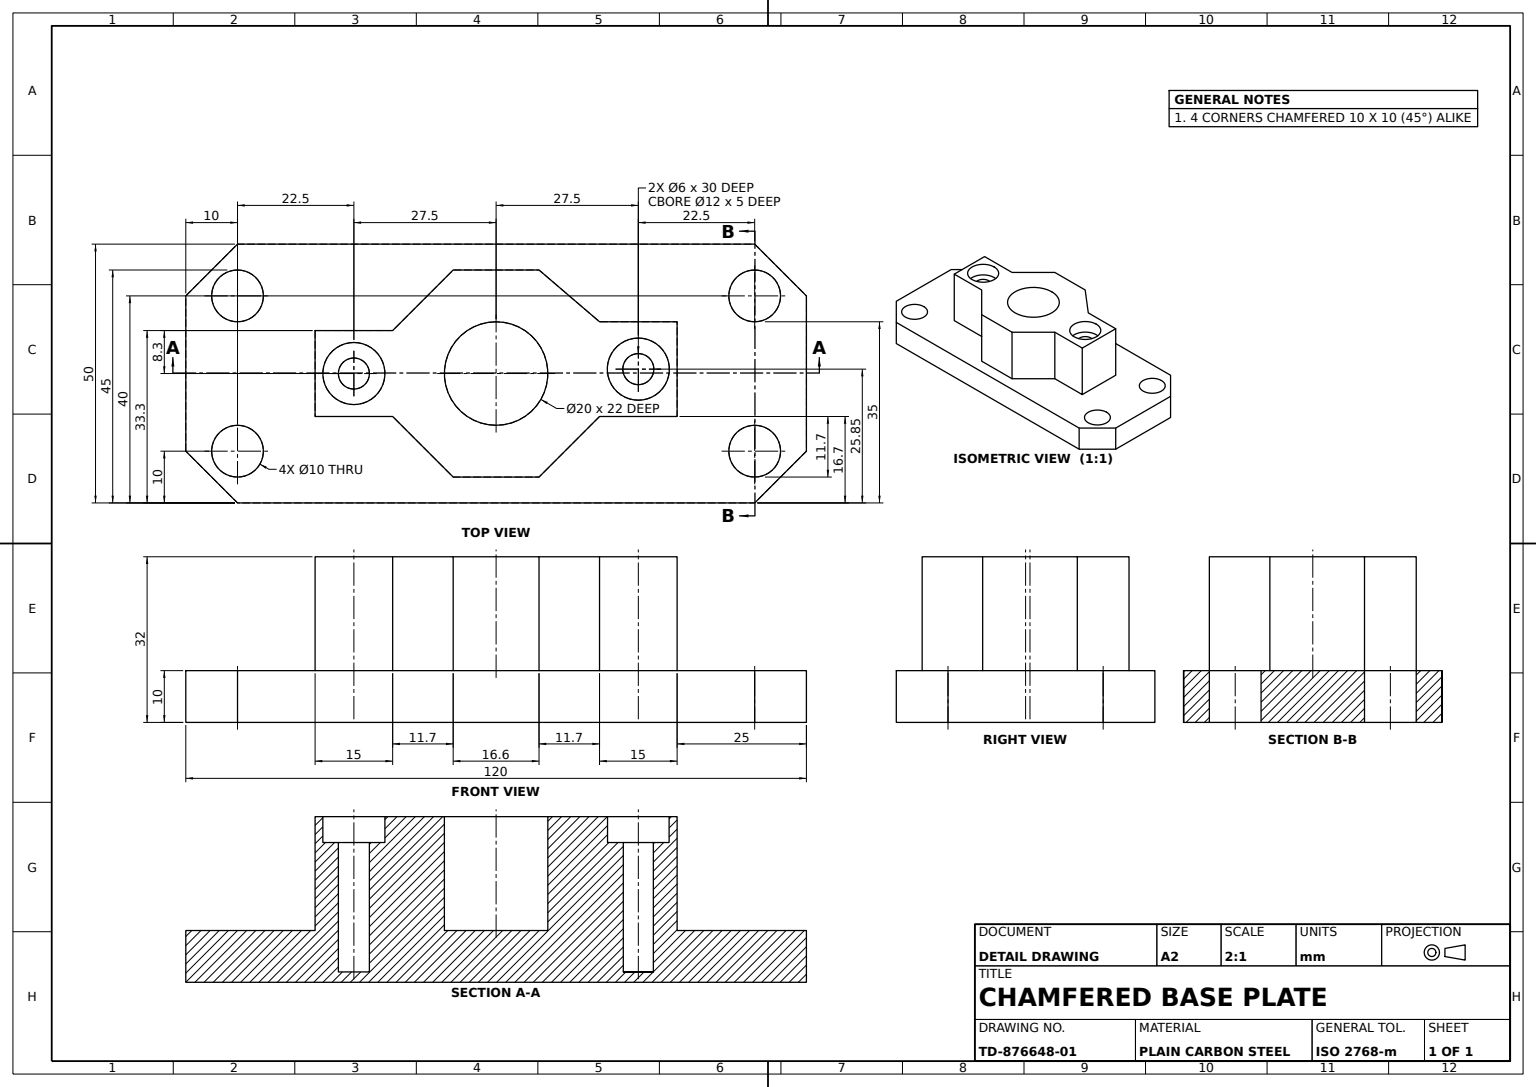
from build123d import *

# Parameters (mm, degrees)
BASE_PLATE_SKETCH_W        = 120
BASE_PLATE_SKETCH_H        = 10
BASE_PLATE_DEPTH           = 50
MOUNTING_HOLES_SKETCH_R    = 5
MOUNTING_HOLES_4X_10_DEPTH = 131.384048104
CENTER_SUPPORT_DEPTH       = 22
CENTER_BORE_SKETCH_R       = 10
CENTER_BORE_20_DEPTH       = 22
SUPPORT_HOLES_SKETCH_R     = 3
SUPPORT_HOLES_2X_6_DEPTH   = 30
COUNTERBORE_SKETCH_R       = 6
COUNTERBORES_2X_12X5_DEPTH = 5
CORNER_CHAMFERS_10MM_SIZE  = 10


with BuildPart() as part:
    # Base Plate Sketch → Base Plate (new body)
    with BuildSketch(Plane.XY):
        with Locations((60, 5)):
            Rectangle(BASE_PLATE_SKETCH_W, BASE_PLATE_SKETCH_H)
    extrude(amount=BASE_PLATE_DEPTH)

    # Mounting Holes Sketch → Mounting Holes 4xØ10 (cut, through all)
    with BuildSketch(Plane(origin=(0, 10, 0), x_dir=(1, 0, 0), z_dir=(0, 1, 0))):
        with Locations(Location((10, -10, 0), (0, 0, 270))):
            Circle(MOUNTING_HOLES_SKETCH_R)
        with Locations(Location((10, -40, 0), (0, 0, 270))):
            Circle(MOUNTING_HOLES_SKETCH_R)
        with Locations(Location((110, -10, 0), (0, 0, 270))):
            Circle(MOUNTING_HOLES_SKETCH_R)
        with Locations(Location((110, -40, 0), (0, 0, 270))):
            Circle(MOUNTING_HOLES_SKETCH_R)
    extrude(amount=-MOUNTING_HOLES_4X_10_DEPTH, mode=Mode.SUBTRACT)

    # Center Support Sketch → Center Support (add)
    with BuildSketch(Plane(origin=(0, 10, 0), x_dir=(1, 0, 0), z_dir=(0, 1, 0))):
        Polygon((25, -16.7), (40, -16.7), (51.7, -5), (68.3, -5), (80, -15), (95, -15), (95, -33.3), (80, -33.3), (68.3, -45), (51.7, -45), (40, -33.3), (25, -33.3), align=None)
    extrude(amount=CENTER_SUPPORT_DEPTH)

    # Center Bore Sketch → Center Bore Ø20 (cut)
    with BuildSketch(Plane(origin=(0, 32, 0), x_dir=(1, 0, 0), z_dir=(0, 1, 0))):
        with Locations(Location((60, -25, 0), (0, 0, 270))):
            Circle(CENTER_BORE_SKETCH_R)
    extrude(amount=-CENTER_BORE_20_DEPTH, mode=Mode.SUBTRACT)

    # Support Holes Sketch → Support Holes 2xØ6 (cut)
    with BuildSketch(Plane(origin=(0, 32, 0), x_dir=(1, 0, 0), z_dir=(0, 1, 0))):
        with Locations(Location((32.5, -25, 0), (0, 0, 270))):
            Circle(SUPPORT_HOLES_SKETCH_R)
        with Locations(Location((87.5, -24.15, 0), (0, 0, 270))):
            Circle(SUPPORT_HOLES_SKETCH_R)
    extrude(amount=-SUPPORT_HOLES_2X_6_DEPTH, mode=Mode.SUBTRACT)

    # Counterbore Sketch → Counterbores 2xØ12x5 (cut)
    with BuildSketch(Plane(origin=(0, 32, 0), x_dir=(1, 0, 0), z_dir=(0, 1, 0))):
        with Locations(Location((32.5, -25, 0), (0, 0, 270))):
            Circle(COUNTERBORE_SKETCH_R)
        with Locations(Location((87.5, -24.15, 0), (0, 0, 270))):
            Circle(COUNTERBORE_SKETCH_R)
    extrude(amount=-COUNTERBORES_2X_12X5_DEPTH, mode=Mode.SUBTRACT)

    # Corner Chamfers 10mm
    corner_chamfers_10mm_edges = [part.edges().sort_by_distance(p)[0] for p in [
        (120, 5, 50),
        (0, 5, 50),
        (120, 5, 0),
        (0, 5, 0),
    ]]
    chamfer(corner_chamfers_10mm_edges, length=CORNER_CHAMFERS_10MM_SIZE)


solid = part.part
